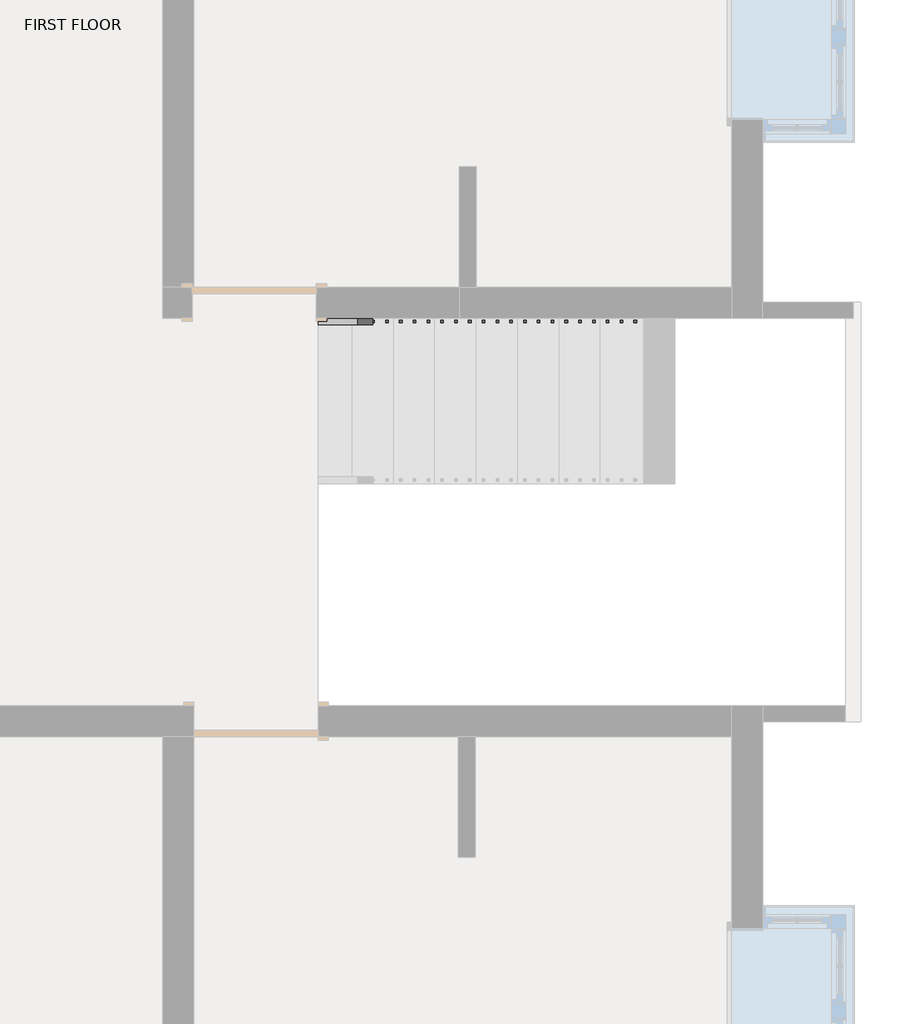
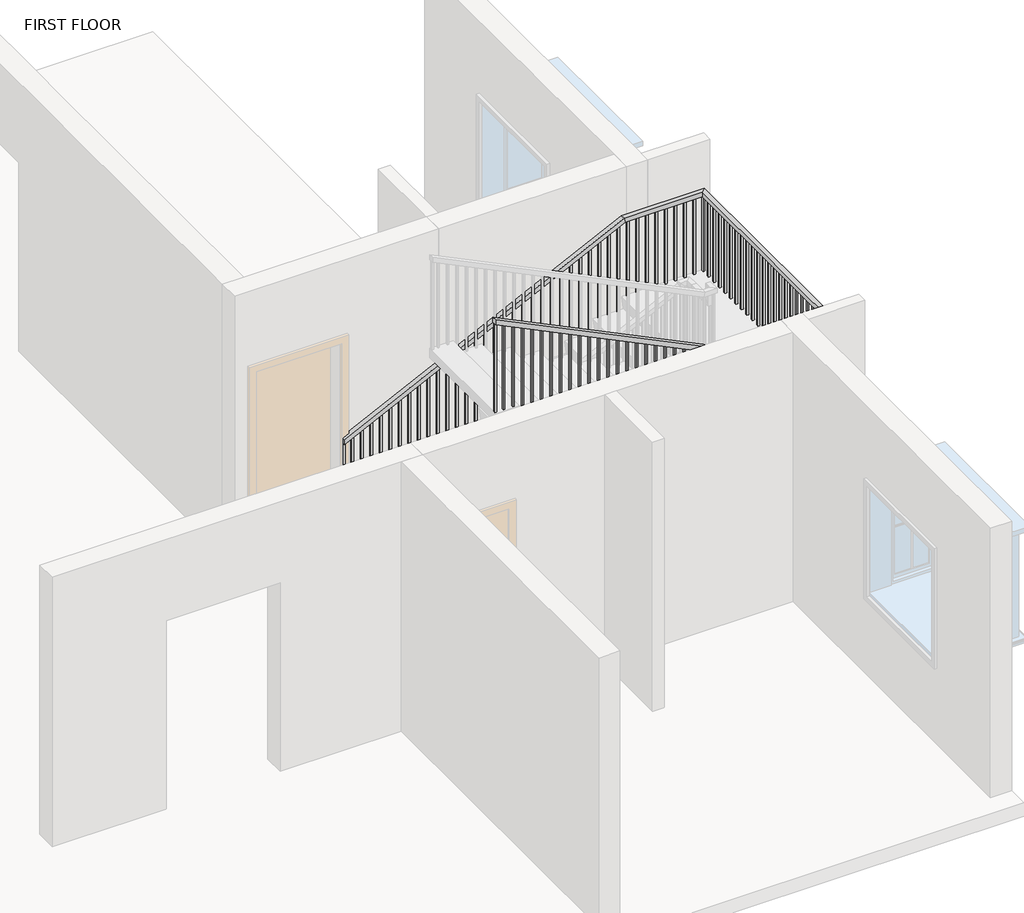
# One storey, part 4 of 6: 1 railing.
"""IFC4 building model written with IfcOpenShell, lengths in millimetres."""

from ifc_helpers import new_model, si_unit, frame, origin, place, context, project, spatial, polyline, outline, extrude, faceted_brep, element, save

model = new_model("IFC4")

# Units and contexts
model_context = context("Model", 3, world=origin())
ifc_project = project(units=[si_unit("LENGTHUNIT", "METRE", prefix="MILLI")], contexts=[model_context])

# Site, building, storey
site = spatial("IfcSite", under=ifc_project)
building = spatial("IfcBuilding", under=site)
storey = spatial("IfcBuildingStorey", under=building, Name="FIRST FLOOR", Elevation=3200.4)

# Railing
placement = place(None, origin())
element("IfcRailing", 1, ObjectType="Handrail - Rectangular", at=placement, inside=storey, context=model_context, shape_type="SolidModel", body=[
    faceted_brep([(3126.2584916, 220.733346, 4260.2727273), (3126.2584916, 220.733346, 4203.7956113), (3126.2584916, 169.933346, 4203.7956113), (3126.2584916, 169.933346, 4260.2727273), (6120.7829507, 220.733346, 5715.0), (6132.4691705, 220.733346, 5664.2), (6132.4691705, 169.933346, 5664.2), (6120.7829507, 169.933346, 5715.0), (7009.1350459, 220.733346, 5715.0), (7009.1350459, 220.733346, 5664.2), (6958.3350459, 169.933346, 5664.2), (6958.3350459, 169.933346, 5715.0), (7009.1350459, -2636.766654, 5715.0), (7009.1350459, -2636.766654, 5664.2), (6958.3350459, -2585.966654, 5664.2), (6958.3350459, -2585.966654, 5715.0), (6420.2353966, -2636.766654, 5715.0), (6408.5491768, -2636.766654, 5664.2), (6408.5491768, -2585.966654, 5664.2), (6420.2353966, -2585.966654, 5715.0), (3126.2584916, -2636.766654, 7315.2), (3126.2584916, -2585.966654, 7315.2), (3126.2584916, -2585.966654, 7258.722884), (3126.2584916, -2636.766654, 7258.722884)], [[[0, 1, 2, 3]], [[1, 0, 4, 5]], [[2, 1, 5, 6]], [[3, 2, 6, 7]], [[0, 3, 7, 4]], [[5, 4, 8, 9]], [[6, 5, 9, 10]], [[7, 6, 10, 11]], [[4, 7, 11, 8]], [[9, 8, 12, 13]], [[10, 9, 13, 14]], [[11, 10, 14, 15]], [[8, 11, 15, 12]], [[13, 12, 16, 17]], [[14, 13, 17, 18]], [[15, 14, 18, 19]], [[12, 15, 19, 16]], [[20, 21, 22, 23]], [[17, 16, 20, 23]], [[18, 17, 23, 22]], [[19, 18, 22, 21]], [[16, 19, 21, 20]]]),
    extrude(outline(polyline([(7215.6077556, 3215.0100459), (6255.3272727, 3215.0100459), (6255.3272727, 3234.0600459), (7206.3533465, 3234.0600459), (7215.6077556, 3215.0100459)])), frame((0.0, -2620.891654, 0.0), z_axis=(0.0, 1.0, 0.0), x_axis=(0.0, 0.0, 1.0)), (0.0, 0.0, 1.0), 19.05),
    extrude(outline(polyline([(7166.2509068, 3316.6100459), (6255.3272727, 3316.6100459), (6255.3272727, 3335.6600459), (7156.9964977, 3335.6600459), (7166.2509068, 3316.6100459)])), frame((0.0, -2620.891654, 0.0), z_axis=(0.0, 1.0, 0.0), x_axis=(0.0, 0.0, 1.0)), (0.0, 0.0, 1.0), 19.05),
    extrude(outline(polyline([(7116.894058, 3418.2100459), (6109.8545455, 3418.2100459), (6109.8545455, 3437.2600459), (7107.6396489, 3437.2600459), (7116.894058, 3418.2100459)])), frame((0.0, -2620.891654, 0.0), z_axis=(0.0, 1.0, 0.0), x_axis=(0.0, 0.0, 1.0)), (0.0, 0.0, 1.0), 19.05),
    extrude(outline(polyline([(7067.5372093, 3519.8100459), (6109.8545455, 3519.8100459), (6109.8545455, 3538.8600459), (7058.2828001, 3538.8600459), (7067.5372093, 3519.8100459)])), frame((0.0, -2620.891654, 0.0), z_axis=(0.0, 1.0, 0.0), x_axis=(0.0, 0.0, 1.0)), (0.0, 0.0, 1.0), 19.05),
    extrude(outline(polyline([(7018.1803605, 3621.4100459), (6109.8545455, 3621.4100459), (6109.8545455, 3640.4600459), (7008.9259513, 3640.4600459), (7018.1803605, 3621.4100459)])), frame((0.0, -2620.891654, 0.0), z_axis=(0.0, 1.0, 0.0), x_axis=(0.0, 0.0, 1.0)), (0.0, 0.0, 1.0), 19.05),
    extrude(outline(polyline([(6968.8235117, 3723.0100459), (5964.3818182, 3723.0100459), (5964.3818182, 3742.0600459), (6959.5691025, 3742.0600459), (6968.8235117, 3723.0100459)])), frame((0.0, -2620.891654, 0.0), z_axis=(0.0, 1.0, 0.0), x_axis=(0.0, 0.0, 1.0)), (0.0, 0.0, 1.0), 19.05),
    extrude(outline(polyline([(6919.4666629, 3824.6100459), (5964.3818182, 3824.6100459), (5964.3818182, 3843.6600459), (6910.2122538, 3843.6600459), (6919.4666629, 3824.6100459)])), frame((0.0, -2620.891654, 0.0), z_axis=(0.0, 1.0, 0.0), x_axis=(0.0, 0.0, 1.0)), (0.0, 0.0, 1.0), 19.05),
    extrude(outline(polyline([(6870.1098141, 3926.2100459), (5964.3818182, 3926.2100459), (5964.3818182, 3945.2600459), (6860.855405, 3945.2600459), (6870.1098141, 3926.2100459)])), frame((0.0, -2620.891654, 0.0), z_axis=(0.0, 1.0, 0.0), x_axis=(0.0, 0.0, 1.0)), (0.0, 0.0, 1.0), 19.05),
    extrude(outline(polyline([(6820.7529653, 4027.8100459), (5818.9090909, 4027.8100459), (5818.9090909, 4046.8600459), (6811.4985562, 4046.8600459), (6820.7529653, 4027.8100459)])), frame((0.0, -2620.891654, 0.0), z_axis=(0.0, 1.0, 0.0), x_axis=(0.0, 0.0, 1.0)), (0.0, 0.0, 1.0), 19.05),
    extrude(outline(polyline([(6771.3961165, 4129.4100459), (5818.9090909, 4129.4100459), (5818.9090909, 4148.4600459), (6762.1417074, 4148.4600459), (6771.3961165, 4129.4100459)])), frame((0.0, -2620.891654, 0.0), z_axis=(0.0, 1.0, 0.0), x_axis=(0.0, 0.0, 1.0)), (0.0, 0.0, 1.0), 19.05),
    extrude(outline(polyline([(6722.0392678, 4231.0100459), (5818.9090909, 4231.0100459), (5818.9090909, 4250.0600459), (6712.7848586, 4250.0600459), (6722.0392678, 4231.0100459)])), frame((0.0, -2620.891654, 0.0), z_axis=(0.0, 1.0, 0.0), x_axis=(0.0, 0.0, 1.0)), (0.0, 0.0, 1.0), 19.05),
    extrude(outline(polyline([(6672.682419, 4332.6100459), (5673.4363636, 4332.6100459), (5673.4363636, 4351.6600459), (6663.4280098, 4351.6600459), (6672.682419, 4332.6100459)])), frame((0.0, -2620.891654, 0.0), z_axis=(0.0, 1.0, 0.0), x_axis=(0.0, 0.0, 1.0)), (0.0, 0.0, 1.0), 19.05),
    extrude(outline(polyline([(6623.3255702, 4434.2100459), (5673.4363636, 4434.2100459), (5673.4363636, 4453.2600459), (6614.071161, 4453.2600459), (6623.3255702, 4434.2100459)])), frame((0.0, -2620.891654, 0.0), z_axis=(0.0, 1.0, 0.0), x_axis=(0.0, 0.0, 1.0)), (0.0, 0.0, 1.0), 19.05),
    extrude(outline(polyline([(6573.9687214, 4535.8100459), (5673.4363636, 4535.8100459), (5673.4363636, 4554.8600459), (6564.7143123, 4554.8600459), (6573.9687214, 4535.8100459)])), frame((0.0, -2620.891654, 0.0), z_axis=(0.0, 1.0, 0.0), x_axis=(0.0, 0.0, 1.0)), (0.0, 0.0, 1.0), 19.05),
    extrude(outline(polyline([(6524.6118726, 4637.4100459), (5527.9636364, 4637.4100459), (5527.9636364, 4656.4600459), (6515.3574635, 4656.4600459), (6524.6118726, 4637.4100459)])), frame((0.0, -2620.891654, 0.0), z_axis=(0.0, 1.0, 0.0), x_axis=(0.0, 0.0, 1.0)), (0.0, 0.0, 1.0), 19.05),
    extrude(outline(polyline([(6475.2550238, 4739.0100459), (5527.9636364, 4739.0100459), (5527.9636364, 4758.0600459), (6466.0006147, 4758.0600459), (6475.2550238, 4739.0100459)])), frame((0.0, -2620.891654, 0.0), z_axis=(0.0, 1.0, 0.0), x_axis=(0.0, 0.0, 1.0)), (0.0, 0.0, 1.0), 19.05),
    extrude(outline(polyline([(6425.8981751, 4840.6100459), (5527.9636364, 4840.6100459), (5527.9636364, 4859.6600459), (6416.6437659, 4859.6600459), (6425.8981751, 4840.6100459)])), frame((0.0, -2620.891654, 0.0), z_axis=(0.0, 1.0, 0.0), x_axis=(0.0, 0.0, 1.0)), (0.0, 0.0, 1.0), 19.05),
    extrude(outline(polyline([(6376.5413263, 4942.2100459), (5382.4909091, 4942.2100459), (5382.4909091, 4961.2600459), (6367.2869171, 4961.2600459), (6376.5413263, 4942.2100459)])), frame((0.0, -2620.891654, 0.0), z_axis=(0.0, 1.0, 0.0), x_axis=(0.0, 0.0, 1.0)), (0.0, 0.0, 1.0), 19.05),
    extrude(outline(polyline([(6327.1844775, 5043.8100459), (5382.4909091, 5043.8100459), (5382.4909091, 5062.8600459), (6317.9300683, 5062.8600459), (6327.1844775, 5043.8100459)])), frame((0.0, -2620.891654, 0.0), z_axis=(0.0, 1.0, 0.0), x_axis=(0.0, 0.0, 1.0)), (0.0, 0.0, 1.0), 19.05),
    extrude(outline(polyline([(6277.8276287, 5145.4100459), (5382.4909091, 5145.4100459), (5382.4909091, 5164.4600459), (6268.5732196, 5164.4600459), (6277.8276287, 5145.4100459)])), frame((0.0, -2620.891654, 0.0), z_axis=(0.0, 1.0, 0.0), x_axis=(0.0, 0.0, 1.0)), (0.0, 0.0, 1.0), 19.05),
    extrude(outline(polyline([(6228.4707799, 5247.0100459), (5237.0181818, 5247.0100459), (5237.0181818, 5266.0600459), (6219.2163708, 5266.0600459), (6228.4707799, 5247.0100459)])), frame((0.0, -2620.891654, 0.0), z_axis=(0.0, 1.0, 0.0), x_axis=(0.0, 0.0, 1.0)), (0.0, 0.0, 1.0), 19.05),
    extrude(outline(polyline([(6179.1139311, 5348.6100459), (5237.0181818, 5348.6100459), (5237.0181818, 5367.6600459), (6169.859522, 5367.6600459), (6179.1139311, 5348.6100459)])), frame((0.0, -2620.891654, 0.0), z_axis=(0.0, 1.0, 0.0), x_axis=(0.0, 0.0, 1.0)), (0.0, 0.0, 1.0), 19.05),
    extrude(outline(polyline([(6129.7570823, 5450.2100459), (5237.0181818, 5450.2100459), (5237.0181818, 5469.2600459), (6120.5026732, 5469.2600459), (6129.7570823, 5450.2100459)])), frame((0.0, -2620.891654, 0.0), z_axis=(0.0, 1.0, 0.0), x_axis=(0.0, 0.0, 1.0)), (0.0, 0.0, 1.0), 19.05),
    extrude(outline(polyline([(6080.4002336, 5551.8100459), (5091.5454545, 5551.8100459), (5091.5454545, 5570.8600459), (6071.1458244, 5570.8600459), (6080.4002336, 5551.8100459)])), frame((0.0, -2620.891654, 0.0), z_axis=(0.0, 1.0, 0.0), x_axis=(0.0, 0.0, 1.0)), (0.0, 0.0, 1.0), 19.05),
    extrude(outline(polyline([(6031.0433848, 5653.4100459), (5091.5454545, 5653.4100459), (5091.5454545, 5672.4600459), (6021.7889756, 5672.4600459), (6031.0433848, 5653.4100459)])), frame((0.0, -2620.891654, 0.0), z_axis=(0.0, 1.0, 0.0), x_axis=(0.0, 0.0, 1.0)), (0.0, 0.0, 1.0), 19.05),
    extrude(outline(polyline([(5981.686536, 5755.0100459), (5091.5454545, 5755.0100459), (5091.5454545, 5774.0600459), (5972.4321268, 5774.0600459), (5981.686536, 5755.0100459)])), frame((0.0, -2620.891654, 0.0), z_axis=(0.0, 1.0, 0.0), x_axis=(0.0, 0.0, 1.0)), (0.0, 0.0, 1.0), 19.05),
    extrude(outline(polyline([(5932.3296872, 5856.6100459), (4946.0727273, 5856.6100459), (4946.0727273, 5875.6600459), (5923.0752781, 5875.6600459), (5932.3296872, 5856.6100459)])), frame((0.0, -2620.891654, 0.0), z_axis=(0.0, 1.0, 0.0), x_axis=(0.0, 0.0, 1.0)), (0.0, 0.0, 1.0), 19.05),
    extrude(outline(polyline([(5882.9728384, 5958.2100459), (4946.0727273, 5958.2100459), (4946.0727273, 5977.2600459), (5873.7184293, 5977.2600459), (5882.9728384, 5958.2100459)])), frame((0.0, -2620.891654, 0.0), z_axis=(0.0, 1.0, 0.0), x_axis=(0.0, 0.0, 1.0)), (0.0, 0.0, 1.0), 19.05),
    extrude(outline(polyline([(5833.6159896, 6059.8100459), (4946.0727273, 6059.8100459), (4946.0727273, 6078.8600459), (5824.3615805, 6078.8600459), (5833.6159896, 6059.8100459)])), frame((0.0, -2620.891654, 0.0), z_axis=(0.0, 1.0, 0.0), x_axis=(0.0, 0.0, 1.0)), (0.0, 0.0, 1.0), 19.05),
    extrude(outline(polyline([(5784.2591409, 6161.4100459), (4800.6, 6161.4100459), (4800.6, 6180.4600459), (5775.0047317, 6180.4600459), (5784.2591409, 6161.4100459)])), frame((0.0, -2620.891654, 0.0), z_axis=(0.0, 1.0, 0.0), x_axis=(0.0, 0.0, 1.0)), (0.0, 0.0, 1.0), 19.05),
    extrude(outline(polyline([(5734.9022921, 6263.0100459), (4800.6, 6263.0100459), (4800.6, 6282.0600459), (5725.6478829, 6282.0600459), (5734.9022921, 6263.0100459)])), frame((0.0, -2620.891654, 0.0), z_axis=(0.0, 1.0, 0.0), x_axis=(0.0, 0.0, 1.0)), (0.0, 0.0, 1.0), 19.05),
    extrude(outline(polyline([(5685.5454433, 6364.6100459), (4800.6, 6364.6100459), (4800.6, 6383.6600459), (5676.2910341, 6383.6600459), (5685.5454433, 6364.6100459)])), frame((0.0, -2620.891654, 0.0), z_axis=(0.0, 1.0, 0.0), x_axis=(0.0, 0.0, 1.0)), (0.0, 0.0, 1.0), 19.05),
    extrude(outline(polyline([(6485.2600459, -2620.891654), (6466.2100459, -2620.891654), (6466.2100459, -2601.841654), (6485.2600459, -2601.841654), (6485.2600459, -2620.891654)])), frame((0.0, 0.0, 4800.6), z_axis=(0.0, 0.0, 1.0), x_axis=(1.0, 0.0, 0.0)), (0.0, 0.0, 1.0), 863.6),
    extrude(outline(polyline([(6586.8600459, -2620.891654), (6567.8100459, -2620.891654), (6567.8100459, -2601.841654), (6586.8600459, -2601.841654), (6586.8600459, -2620.891654)])), frame((0.0, 0.0, 4800.6), z_axis=(0.0, 0.0, 1.0), x_axis=(1.0, 0.0, 0.0)), (0.0, 0.0, 1.0), 863.6),
    extrude(outline(polyline([(6688.4600459, -2620.891654), (6669.4100459, -2620.891654), (6669.4100459, -2601.841654), (6688.4600459, -2601.841654), (6688.4600459, -2620.891654)])), frame((0.0, 0.0, 4800.6), z_axis=(0.0, 0.0, 1.0), x_axis=(1.0, 0.0, 0.0)), (0.0, 0.0, 1.0), 863.6),
    extrude(outline(polyline([(6790.0600459, -2620.891654), (6771.0100459, -2620.891654), (6771.0100459, -2601.841654), (6790.0600459, -2601.841654), (6790.0600459, -2620.891654)])), frame((0.0, 0.0, 4800.6), z_axis=(0.0, 0.0, 1.0), x_axis=(1.0, 0.0, 0.0)), (0.0, 0.0, 1.0), 863.6),
    extrude(outline(polyline([(6891.6600459, -2620.891654), (6872.6100459, -2620.891654), (6872.6100459, -2601.841654), (6891.6600459, -2601.841654), (6891.6600459, -2620.891654)])), frame((0.0, 0.0, 4800.6), z_axis=(0.0, 0.0, 1.0), x_axis=(1.0, 0.0, 0.0)), (0.0, 0.0, 1.0), 863.6),
    extrude(outline(polyline([(6993.2600459, -2538.341654), (6993.2600459, -2557.391654), (6974.2100459, -2557.391654), (6974.2100459, -2538.341654), (6993.2600459, -2538.341654)])), frame((0.0, 0.0, 4800.6), z_axis=(0.0, 0.0, 1.0), x_axis=(1.0, 0.0, 0.0)), (0.0, 0.0, 1.0), 863.6),
    extrude(outline(polyline([(6993.2600459, -2436.741654), (6993.2600459, -2455.791654), (6974.2100459, -2455.791654), (6974.2100459, -2436.741654), (6993.2600459, -2436.741654)])), frame((0.0, 0.0, 4800.6), z_axis=(0.0, 0.0, 1.0), x_axis=(1.0, 0.0, 0.0)), (0.0, 0.0, 1.0), 863.6),
    extrude(outline(polyline([(6993.2600459, -2335.141654), (6993.2600459, -2354.191654), (6974.2100459, -2354.191654), (6974.2100459, -2335.141654), (6993.2600459, -2335.141654)])), frame((0.0, 0.0, 4800.6), z_axis=(0.0, 0.0, 1.0), x_axis=(1.0, 0.0, 0.0)), (0.0, 0.0, 1.0), 863.6),
    extrude(outline(polyline([(6993.2600459, -2233.541654), (6993.2600459, -2252.591654), (6974.2100459, -2252.591654), (6974.2100459, -2233.541654), (6993.2600459, -2233.541654)])), frame((0.0, 0.0, 4800.6), z_axis=(0.0, 0.0, 1.0), x_axis=(1.0, 0.0, 0.0)), (0.0, 0.0, 1.0), 863.6),
    extrude(outline(polyline([(6993.2600459, -2131.941654), (6993.2600459, -2150.991654), (6974.2100459, -2150.991654), (6974.2100459, -2131.941654), (6993.2600459, -2131.941654)])), frame((0.0, 0.0, 4800.6), z_axis=(0.0, 0.0, 1.0), x_axis=(1.0, 0.0, 0.0)), (0.0, 0.0, 1.0), 863.6),
    extrude(outline(polyline([(6993.2600459, -2030.341654), (6993.2600459, -2049.391654), (6974.2100459, -2049.391654), (6974.2100459, -2030.341654), (6993.2600459, -2030.341654)])), frame((0.0, 0.0, 4800.6), z_axis=(0.0, 0.0, 1.0), x_axis=(1.0, 0.0, 0.0)), (0.0, 0.0, 1.0), 863.6),
    extrude(outline(polyline([(6993.2600459, -1928.741654), (6993.2600459, -1947.791654), (6974.2100459, -1947.791654), (6974.2100459, -1928.741654), (6993.2600459, -1928.741654)])), frame((0.0, 0.0, 4800.6), z_axis=(0.0, 0.0, 1.0), x_axis=(1.0, 0.0, 0.0)), (0.0, 0.0, 1.0), 863.6),
    extrude(outline(polyline([(6993.2600459, -1827.141654), (6993.2600459, -1846.191654), (6974.2100459, -1846.191654), (6974.2100459, -1827.141654), (6993.2600459, -1827.141654)])), frame((0.0, 0.0, 4800.6), z_axis=(0.0, 0.0, 1.0), x_axis=(1.0, 0.0, 0.0)), (0.0, 0.0, 1.0), 863.6),
    extrude(outline(polyline([(6993.2600459, -1725.541654), (6993.2600459, -1744.591654), (6974.2100459, -1744.591654), (6974.2100459, -1725.541654), (6993.2600459, -1725.541654)])), frame((0.0, 0.0, 4800.6), z_axis=(0.0, 0.0, 1.0), x_axis=(1.0, 0.0, 0.0)), (0.0, 0.0, 1.0), 863.6),
    extrude(outline(polyline([(6993.2600459, -1623.941654), (6993.2600459, -1642.991654), (6974.2100459, -1642.991654), (6974.2100459, -1623.941654), (6993.2600459, -1623.941654)])), frame((0.0, 0.0, 4800.6), z_axis=(0.0, 0.0, 1.0), x_axis=(1.0, 0.0, 0.0)), (0.0, 0.0, 1.0), 863.6),
    extrude(outline(polyline([(6993.2600459, -1522.341654), (6993.2600459, -1541.391654), (6974.2100459, -1541.391654), (6974.2100459, -1522.341654), (6993.2600459, -1522.341654)])), frame((0.0, 0.0, 4800.6), z_axis=(0.0, 0.0, 1.0), x_axis=(1.0, 0.0, 0.0)), (0.0, 0.0, 1.0), 863.6),
    extrude(outline(polyline([(6993.2600459, -1420.741654), (6993.2600459, -1439.791654), (6974.2100459, -1439.791654), (6974.2100459, -1420.741654), (6993.2600459, -1420.741654)])), frame((0.0, 0.0, 4800.6), z_axis=(0.0, 0.0, 1.0), x_axis=(1.0, 0.0, 0.0)), (0.0, 0.0, 1.0), 863.6),
    extrude(outline(polyline([(6993.2600459, -1319.141654), (6993.2600459, -1338.191654), (6974.2100459, -1338.191654), (6974.2100459, -1319.141654), (6993.2600459, -1319.141654)])), frame((0.0, 0.0, 4800.6), z_axis=(0.0, 0.0, 1.0), x_axis=(1.0, 0.0, 0.0)), (0.0, 0.0, 1.0), 863.6),
    extrude(outline(polyline([(6993.2600459, -1217.541654), (6993.2600459, -1236.591654), (6974.2100459, -1236.591654), (6974.2100459, -1217.541654), (6993.2600459, -1217.541654)])), frame((0.0, 0.0, 4800.6), z_axis=(0.0, 0.0, 1.0), x_axis=(1.0, 0.0, 0.0)), (0.0, 0.0, 1.0), 863.6),
    extrude(outline(polyline([(6993.2600459, -1115.941654), (6993.2600459, -1134.991654), (6974.2100459, -1134.991654), (6974.2100459, -1115.941654), (6993.2600459, -1115.941654)])), frame((0.0, 0.0, 4800.6), z_axis=(0.0, 0.0, 1.0), x_axis=(1.0, 0.0, 0.0)), (0.0, 0.0, 1.0), 863.6),
    extrude(outline(polyline([(6993.2600459, -1014.341654), (6993.2600459, -1033.391654), (6974.2100459, -1033.391654), (6974.2100459, -1014.341654), (6993.2600459, -1014.341654)])), frame((0.0, 0.0, 4800.6), z_axis=(0.0, 0.0, 1.0), x_axis=(1.0, 0.0, 0.0)), (0.0, 0.0, 1.0), 863.6),
    extrude(outline(polyline([(6993.2600459, -912.741654), (6993.2600459, -931.791654), (6974.2100459, -931.791654), (6974.2100459, -912.741654), (6993.2600459, -912.741654)])), frame((0.0, 0.0, 4800.6), z_axis=(0.0, 0.0, 1.0), x_axis=(1.0, 0.0, 0.0)), (0.0, 0.0, 1.0), 863.6),
    extrude(outline(polyline([(6993.2600459, -811.141654), (6993.2600459, -830.191654), (6974.2100459, -830.191654), (6974.2100459, -811.141654), (6993.2600459, -811.141654)])), frame((0.0, 0.0, 4800.6), z_axis=(0.0, 0.0, 1.0), x_axis=(1.0, 0.0, 0.0)), (0.0, 0.0, 1.0), 863.6),
    extrude(outline(polyline([(6993.2600459, -709.541654), (6993.2600459, -728.591654), (6974.2100459, -728.591654), (6974.2100459, -709.541654), (6993.2600459, -709.541654)])), frame((0.0, 0.0, 4800.6), z_axis=(0.0, 0.0, 1.0), x_axis=(1.0, 0.0, 0.0)), (0.0, 0.0, 1.0), 863.6),
    extrude(outline(polyline([(6993.2600459, -607.941654), (6993.2600459, -626.991654), (6974.2100459, -626.991654), (6974.2100459, -607.941654), (6993.2600459, -607.941654)])), frame((0.0, 0.0, 4800.6), z_axis=(0.0, 0.0, 1.0), x_axis=(1.0, 0.0, 0.0)), (0.0, 0.0, 1.0), 863.6),
    extrude(outline(polyline([(6993.2600459, -506.341654), (6993.2600459, -525.391654), (6974.2100459, -525.391654), (6974.2100459, -506.341654), (6993.2600459, -506.341654)])), frame((0.0, 0.0, 4800.6), z_axis=(0.0, 0.0, 1.0), x_axis=(1.0, 0.0, 0.0)), (0.0, 0.0, 1.0), 863.6),
    extrude(outline(polyline([(6993.2600459, -404.741654), (6993.2600459, -423.791654), (6974.2100459, -423.791654), (6974.2100459, -404.741654), (6993.2600459, -404.741654)])), frame((0.0, 0.0, 4800.6), z_axis=(0.0, 0.0, 1.0), x_axis=(1.0, 0.0, 0.0)), (0.0, 0.0, 1.0), 863.6),
    extrude(outline(polyline([(6993.2600459, -303.141654), (6993.2600459, -322.191654), (6974.2100459, -322.191654), (6974.2100459, -303.141654), (6993.2600459, -303.141654)])), frame((0.0, 0.0, 4800.6), z_axis=(0.0, 0.0, 1.0), x_axis=(1.0, 0.0, 0.0)), (0.0, 0.0, 1.0), 863.6),
    extrude(outline(polyline([(6993.2600459, -201.541654), (6993.2600459, -220.591654), (6974.2100459, -220.591654), (6974.2100459, -201.541654), (6993.2600459, -201.541654)])), frame((0.0, 0.0, 4800.6), z_axis=(0.0, 0.0, 1.0), x_axis=(1.0, 0.0, 0.0)), (0.0, 0.0, 1.0), 863.6),
    extrude(outline(polyline([(6993.2600459, -99.941654), (6993.2600459, -118.991654), (6974.2100459, -118.991654), (6974.2100459, -99.941654), (6993.2600459, -99.941654)])), frame((0.0, 0.0, 4800.6), z_axis=(0.0, 0.0, 1.0), x_axis=(1.0, 0.0, 0.0)), (0.0, 0.0, 1.0), 863.6),
    extrude(outline(polyline([(6993.2600459, 1.658346), (6993.2600459, -17.391654), (6974.2100459, -17.391654), (6974.2100459, 1.658346), (6993.2600459, 1.658346)])), frame((0.0, 0.0, 4800.6), z_axis=(0.0, 0.0, 1.0), x_axis=(1.0, 0.0, 0.0)), (0.0, 0.0, 1.0), 863.6),
    extrude(outline(polyline([(6993.2600459, 103.258346), (6993.2600459, 84.208346), (6974.2100459, 84.208346), (6974.2100459, 103.258346), (6993.2600459, 103.258346)])), frame((0.0, 0.0, 4800.6), z_axis=(0.0, 0.0, 1.0), x_axis=(1.0, 0.0, 0.0)), (0.0, 0.0, 1.0), 863.6),
    extrude(outline(polyline([(6875.9334916, 204.858346), (6894.9834916, 204.858346), (6894.9834916, 185.808346), (6875.9334916, 185.808346), (6875.9334916, 204.858346)])), frame((0.0, 0.0, 4800.6), z_axis=(0.0, 0.0, 1.0), x_axis=(1.0, 0.0, 0.0)), (0.0, 0.0, 1.0), 863.6),
    extrude(outline(polyline([(6774.3334916, 204.858346), (6793.3834916, 204.858346), (6793.3834916, 185.808346), (6774.3334916, 185.808346), (6774.3334916, 204.858346)])), frame((0.0, 0.0, 4800.6), z_axis=(0.0, 0.0, 1.0), x_axis=(1.0, 0.0, 0.0)), (0.0, 0.0, 1.0), 863.6),
    extrude(outline(polyline([(6672.7334916, 204.858346), (6691.7834916, 204.858346), (6691.7834916, 185.808346), (6672.7334916, 185.808346), (6672.7334916, 204.858346)])), frame((0.0, 0.0, 4800.6), z_axis=(0.0, 0.0, 1.0), x_axis=(1.0, 0.0, 0.0)), (0.0, 0.0, 1.0), 863.6),
    extrude(outline(polyline([(6571.1334916, 204.858346), (6590.1834916, 204.858346), (6590.1834916, 185.808346), (6571.1334916, 185.808346), (6571.1334916, 204.858346)])), frame((0.0, 0.0, 4800.6), z_axis=(0.0, 0.0, 1.0), x_axis=(1.0, 0.0, 0.0)), (0.0, 0.0, 1.0), 863.6),
    extrude(outline(polyline([(6469.5334916, 204.858346), (6488.5834916, 204.858346), (6488.5834916, 185.808346), (6469.5334916, 185.808346), (6469.5334916, 204.858346)])), frame((0.0, 0.0, 4800.6), z_axis=(0.0, 0.0, 1.0), x_axis=(1.0, 0.0, 0.0)), (0.0, 0.0, 1.0), 863.6),
    extrude(outline(polyline([(6367.9334916, 204.858346), (6386.9834916, 204.858346), (6386.9834916, 185.808346), (6367.9334916, 185.808346), (6367.9334916, 204.858346)])), frame((0.0, 0.0, 4800.6), z_axis=(0.0, 0.0, 1.0), x_axis=(1.0, 0.0, 0.0)), (0.0, 0.0, 1.0), 863.6),
    extrude(outline(polyline([(6266.3334916, 204.858346), (6285.3834916, 204.858346), (6285.3834916, 185.808346), (6266.3334916, 185.808346), (6266.3334916, 204.858346)])), frame((0.0, 0.0, 4800.6), z_axis=(0.0, 0.0, 1.0), x_axis=(1.0, 0.0, 0.0)), (0.0, 0.0, 1.0), 863.6),
    extrude(outline(polyline([(6164.7334916, 204.858346), (6183.7834916, 204.858346), (6183.7834916, 185.808346), (6164.7334916, 185.808346), (6164.7334916, 204.858346)])), frame((0.0, 0.0, 4800.6), z_axis=(0.0, 0.0, 1.0), x_axis=(1.0, 0.0, 0.0)), (0.0, 0.0, 1.0), 863.6),
    extrude(outline(polyline([(5630.5170215, 6063.1334916), (4655.1272727, 6063.1334916), (4655.1272727, 6082.1834916), (5639.7714306, 6082.1834916), (5630.5170215, 6063.1334916)])), frame((0.0, 185.808346, 0.0), z_axis=(0.0, 1.0, 0.0), x_axis=(0.0, 0.0, 1.0)), (0.0, 0.0, 1.0), 19.05),
    extrude(outline(polyline([(5581.1601727, 5961.5334916), (4655.1272727, 5961.5334916), (4655.1272727, 5980.5834916), (5590.4145818, 5980.5834916), (5581.1601727, 5961.5334916)])), frame((0.0, 185.808346, 0.0), z_axis=(0.0, 1.0, 0.0), x_axis=(0.0, 0.0, 1.0)), (0.0, 0.0, 1.0), 19.05),
    extrude(outline(polyline([(5531.8033239, 5859.9334916), (4655.1272727, 5859.9334916), (4655.1272727, 5878.9834916), (5541.057733, 5878.9834916), (5531.8033239, 5859.9334916)])), frame((0.0, 185.808346, 0.0), z_axis=(0.0, 1.0, 0.0), x_axis=(0.0, 0.0, 1.0)), (0.0, 0.0, 1.0), 19.05),
    extrude(outline(polyline([(5482.4464751, 5758.3334916), (4509.6545455, 5758.3334916), (4509.6545455, 5777.3834916), (5491.7008843, 5777.3834916), (5482.4464751, 5758.3334916)])), frame((0.0, 185.808346, 0.0), z_axis=(0.0, 1.0, 0.0), x_axis=(0.0, 0.0, 1.0)), (0.0, 0.0, 1.0), 19.05),
    extrude(outline(polyline([(5433.0896263, 5656.7334916), (4509.6545455, 5656.7334916), (4509.6545455, 5675.7834916), (5442.3440355, 5675.7834916), (5433.0896263, 5656.7334916)])), frame((0.0, 185.808346, 0.0), z_axis=(0.0, 1.0, 0.0), x_axis=(0.0, 0.0, 1.0)), (0.0, 0.0, 1.0), 19.05),
    extrude(outline(polyline([(5383.7327775, 5555.1334916), (4509.6545455, 5555.1334916), (4509.6545455, 5574.1834916), (5392.9871867, 5574.1834916), (5383.7327775, 5555.1334916)])), frame((0.0, 185.808346, 0.0), z_axis=(0.0, 1.0, 0.0), x_axis=(0.0, 0.0, 1.0)), (0.0, 0.0, 1.0), 19.05),
    extrude(outline(polyline([(5334.3759288, 5453.5334916), (4364.1818182, 5453.5334916), (4364.1818182, 5472.5834916), (5343.6303379, 5472.5834916), (5334.3759288, 5453.5334916)])), frame((0.0, 185.808346, 0.0), z_axis=(0.0, 1.0, 0.0), x_axis=(0.0, 0.0, 1.0)), (0.0, 0.0, 1.0), 19.05),
    extrude(outline(polyline([(5285.01908, 5351.9334916), (4364.1818182, 5351.9334916), (4364.1818182, 5370.9834916), (5294.2734891, 5370.9834916), (5285.01908, 5351.9334916)])), frame((0.0, 185.808346, 0.0), z_axis=(0.0, 1.0, 0.0), x_axis=(0.0, 0.0, 1.0)), (0.0, 0.0, 1.0), 19.05),
    extrude(outline(polyline([(5235.6622312, 5250.3334916), (4364.1818182, 5250.3334916), (4364.1818182, 5269.3834916), (5244.9166403, 5269.3834916), (5235.6622312, 5250.3334916)])), frame((0.0, 185.808346, 0.0), z_axis=(0.0, 1.0, 0.0), x_axis=(0.0, 0.0, 1.0)), (0.0, 0.0, 1.0), 19.05),
    extrude(outline(polyline([(5186.3053824, 5148.7334916), (4218.7090909, 5148.7334916), (4218.7090909, 5167.7834916), (5195.5597915, 5167.7834916), (5186.3053824, 5148.7334916)])), frame((0.0, 185.808346, 0.0), z_axis=(0.0, 1.0, 0.0), x_axis=(0.0, 0.0, 1.0)), (0.0, 0.0, 1.0), 19.05),
    extrude(outline(polyline([(5136.9485336, 5047.1334916), (4218.7090909, 5047.1334916), (4218.7090909, 5066.1834916), (5146.2029428, 5066.1834916), (5136.9485336, 5047.1334916)])), frame((0.0, 185.808346, 0.0), z_axis=(0.0, 1.0, 0.0), x_axis=(0.0, 0.0, 1.0)), (0.0, 0.0, 1.0), 19.05),
    extrude(outline(polyline([(5087.5916848, 4945.5334916), (4218.7090909, 4945.5334916), (4218.7090909, 4964.5834916), (5096.846094, 4964.5834916), (5087.5916848, 4945.5334916)])), frame((0.0, 185.808346, 0.0), z_axis=(0.0, 1.0, 0.0), x_axis=(0.0, 0.0, 1.0)), (0.0, 0.0, 1.0), 19.05),
    extrude(outline(polyline([(5038.234836, 4843.9334916), (4073.2363636, 4843.9334916), (4073.2363636, 4862.9834916), (5047.4892452, 4862.9834916), (5038.234836, 4843.9334916)])), frame((0.0, 185.808346, 0.0), z_axis=(0.0, 1.0, 0.0), x_axis=(0.0, 0.0, 1.0)), (0.0, 0.0, 1.0), 19.05),
    extrude(outline(polyline([(4988.8779873, 4742.3334916), (4073.2363636, 4742.3334916), (4073.2363636, 4761.3834916), (4998.1323964, 4761.3834916), (4988.8779873, 4742.3334916)])), frame((0.0, 185.808346, 0.0), z_axis=(0.0, 1.0, 0.0), x_axis=(0.0, 0.0, 1.0)), (0.0, 0.0, 1.0), 19.05),
    extrude(outline(polyline([(4939.5211385, 4640.7334916), (4073.2363636, 4640.7334916), (4073.2363636, 4659.7834916), (4948.7755476, 4659.7834916), (4939.5211385, 4640.7334916)])), frame((0.0, 185.808346, 0.0), z_axis=(0.0, 1.0, 0.0), x_axis=(0.0, 0.0, 1.0)), (0.0, 0.0, 1.0), 19.05),
    extrude(outline(polyline([(4890.1642897, 4539.1334916), (3927.7636364, 4539.1334916), (3927.7636364, 4558.1834916), (4899.4186988, 4558.1834916), (4890.1642897, 4539.1334916)])), frame((0.0, 185.808346, 0.0), z_axis=(0.0, 1.0, 0.0), x_axis=(0.0, 0.0, 1.0)), (0.0, 0.0, 1.0), 19.05),
    extrude(outline(polyline([(4840.8074409, 4437.5334916), (3927.7636364, 4437.5334916), (3927.7636364, 4456.5834916), (4850.0618501, 4456.5834916), (4840.8074409, 4437.5334916)])), frame((0.0, 185.808346, 0.0), z_axis=(0.0, 1.0, 0.0), x_axis=(0.0, 0.0, 1.0)), (0.0, 0.0, 1.0), 19.05),
    extrude(outline(polyline([(4791.4505921, 4335.9334916), (3927.7636364, 4335.9334916), (3927.7636364, 4354.9834916), (4800.7050013, 4354.9834916), (4791.4505921, 4335.9334916)])), frame((0.0, 185.808346, 0.0), z_axis=(0.0, 1.0, 0.0), x_axis=(0.0, 0.0, 1.0)), (0.0, 0.0, 1.0), 19.05),
    extrude(outline(polyline([(4742.0937433, 4234.3334916), (3782.2909091, 4234.3334916), (3782.2909091, 4253.3834916), (4751.3481525, 4253.3834916), (4742.0937433, 4234.3334916)])), frame((0.0, 185.808346, 0.0), z_axis=(0.0, 1.0, 0.0), x_axis=(0.0, 0.0, 1.0)), (0.0, 0.0, 1.0), 19.05),
    extrude(outline(polyline([(4692.7368946, 4132.7334916), (3782.2909091, 4132.7334916), (3782.2909091, 4151.7834916), (4701.9913037, 4151.7834916), (4692.7368946, 4132.7334916)])), frame((0.0, 185.808346, 0.0), z_axis=(0.0, 1.0, 0.0), x_axis=(0.0, 0.0, 1.0)), (0.0, 0.0, 1.0), 19.05),
    extrude(outline(polyline([(4643.3800458, 4031.1334916), (3782.2909091, 4031.1334916), (3782.2909091, 4050.1834916), (4652.6344549, 4050.1834916), (4643.3800458, 4031.1334916)])), frame((0.0, 185.808346, 0.0), z_axis=(0.0, 1.0, 0.0), x_axis=(0.0, 0.0, 1.0)), (0.0, 0.0, 1.0), 19.05),
    extrude(outline(polyline([(4594.023197, 3929.5334916), (3636.8181818, 3929.5334916), (3636.8181818, 3948.5834916), (4603.2776061, 3948.5834916), (4594.023197, 3929.5334916)])), frame((0.0, 185.808346, 0.0), z_axis=(0.0, 1.0, 0.0), x_axis=(0.0, 0.0, 1.0)), (0.0, 0.0, 1.0), 19.05),
    extrude(outline(polyline([(4544.6663482, 3827.9334916), (3636.8181818, 3827.9334916), (3636.8181818, 3846.9834916), (4553.9207573, 3846.9834916), (4544.6663482, 3827.9334916)])), frame((0.0, 185.808346, 0.0), z_axis=(0.0, 1.0, 0.0), x_axis=(0.0, 0.0, 1.0)), (0.0, 0.0, 1.0), 19.05),
    extrude(outline(polyline([(4495.3094994, 3726.3334916), (3636.8181818, 3726.3334916), (3636.8181818, 3745.3834916), (4504.5639086, 3745.3834916), (4495.3094994, 3726.3334916)])), frame((0.0, 185.808346, 0.0), z_axis=(0.0, 1.0, 0.0), x_axis=(0.0, 0.0, 1.0)), (0.0, 0.0, 1.0), 19.05),
    extrude(outline(polyline([(4445.9526506, 3624.7334916), (3491.3454545, 3624.7334916), (3491.3454545, 3643.7834916), (4455.2070598, 3643.7834916), (4445.9526506, 3624.7334916)])), frame((0.0, 185.808346, 0.0), z_axis=(0.0, 1.0, 0.0), x_axis=(0.0, 0.0, 1.0)), (0.0, 0.0, 1.0), 19.05),
    extrude(outline(polyline([(4396.5958018, 3523.1334916), (3491.3454545, 3523.1334916), (3491.3454545, 3542.1834916), (4405.850211, 3542.1834916), (4396.5958018, 3523.1334916)])), frame((0.0, 185.808346, 0.0), z_axis=(0.0, 1.0, 0.0), x_axis=(0.0, 0.0, 1.0)), (0.0, 0.0, 1.0), 19.05),
    extrude(outline(polyline([(4347.2389531, 3421.5334916), (3491.3454545, 3421.5334916), (3491.3454545, 3440.5834916), (4356.4933622, 3440.5834916), (4347.2389531, 3421.5334916)])), frame((0.0, 185.808346, 0.0), z_axis=(0.0, 1.0, 0.0), x_axis=(0.0, 0.0, 1.0)), (0.0, 0.0, 1.0), 19.05),
    extrude(outline(polyline([(4297.8821043, 3319.9334916), (3345.8727273, 3319.9334916), (3345.8727273, 3338.9834916), (4307.1365134, 3338.9834916), (4297.8821043, 3319.9334916)])), frame((0.0, 185.808346, 0.0), z_axis=(0.0, 1.0, 0.0), x_axis=(0.0, 0.0, 1.0)), (0.0, 0.0, 1.0), 19.05),
    extrude(outline(polyline([(4248.5252555, 3218.3334916), (3345.8727273, 3218.3334916), (3345.8727273, 3237.3834916), (4257.7796646, 3237.3834916), (4248.5252555, 3218.3334916)])), frame((0.0, 185.808346, 0.0), z_axis=(0.0, 1.0, 0.0), x_axis=(0.0, 0.0, 1.0)), (0.0, 0.0, 1.0), 19.05),
    extrude(outline(polyline([(6993.2600459, -2601.841654), (6993.2600459, -2620.891654), (6974.2100459, -2620.891654), (6974.2100459, -2601.841654), (6993.2600459, -2601.841654)])), frame((0.0, 0.0, 4800.6), z_axis=(0.0, 0.0, 1.0), x_axis=(1.0, 0.0, 0.0)), (0.0, 0.0, 1.0), 863.6),
    extrude(outline(polyline([(6974.2100459, 204.858346), (6993.2600459, 204.858346), (6993.2600459, 185.808346), (6974.2100459, 185.808346), (6974.2100459, 204.858346)])), frame((0.0, 0.0, 4800.6), z_axis=(0.0, 0.0, 1.0), x_axis=(1.0, 0.0, 0.0)), (0.0, 0.0, 1.0), 863.6),
    extrude(outline(polyline([(7258.722884, 3126.2584916), (6255.3272727, 3126.2584916), (6255.3272727, 3145.3084916), (7249.4684749, 3145.3084916), (7258.722884, 3126.2584916)])), frame((0.0, -2620.891654, 0.0), z_axis=(0.0, 1.0, 0.0), x_axis=(0.0, 0.0, 1.0)), (0.0, 0.0, 1.0), 19.05),
    extrude(outline(polyline([(4203.7956113, 3126.2584916), (3345.8727273, 3126.2584916), (3345.8727273, 3145.3084916), (4213.0500204, 3145.3084916), (4203.7956113, 3126.2584916)])), frame((0.0, 185.808346, 0.0), z_axis=(0.0, 1.0, 0.0), x_axis=(0.0, 0.0, 1.0)), (0.0, 0.0, 1.0), 19.05),
])

save(model, "model.ifc")

# Revit data of these elements
# Type "Handrail - Rectangular"
#   Assembly Code = "C2010400"
#   built-in parameter 1008612 = 0.0416667 (stored number, unit not read)
#   built-in parameter 1008611 = 0.0416667 (stored number, unit not read)
#   built-in parameter 1008609 = 0.333333 (stored number, unit not read)
#   built-in parameter 1008604 = 0.166667 (stored number, unit not read)
#   built-in parameter 1008603 = 0.166667 (stored number, unit not read)
#   Railing Height = 3' - 0"
#   built-in parameter 1008630 = 2
#   built-in parameter 1008610 = 2
#   built-in parameter 1008618 = Baluster - Square : 3/4"
# Element 1 (IfcRailing, "Handrail - Rectangular")
#   Phase Created = New Construction
